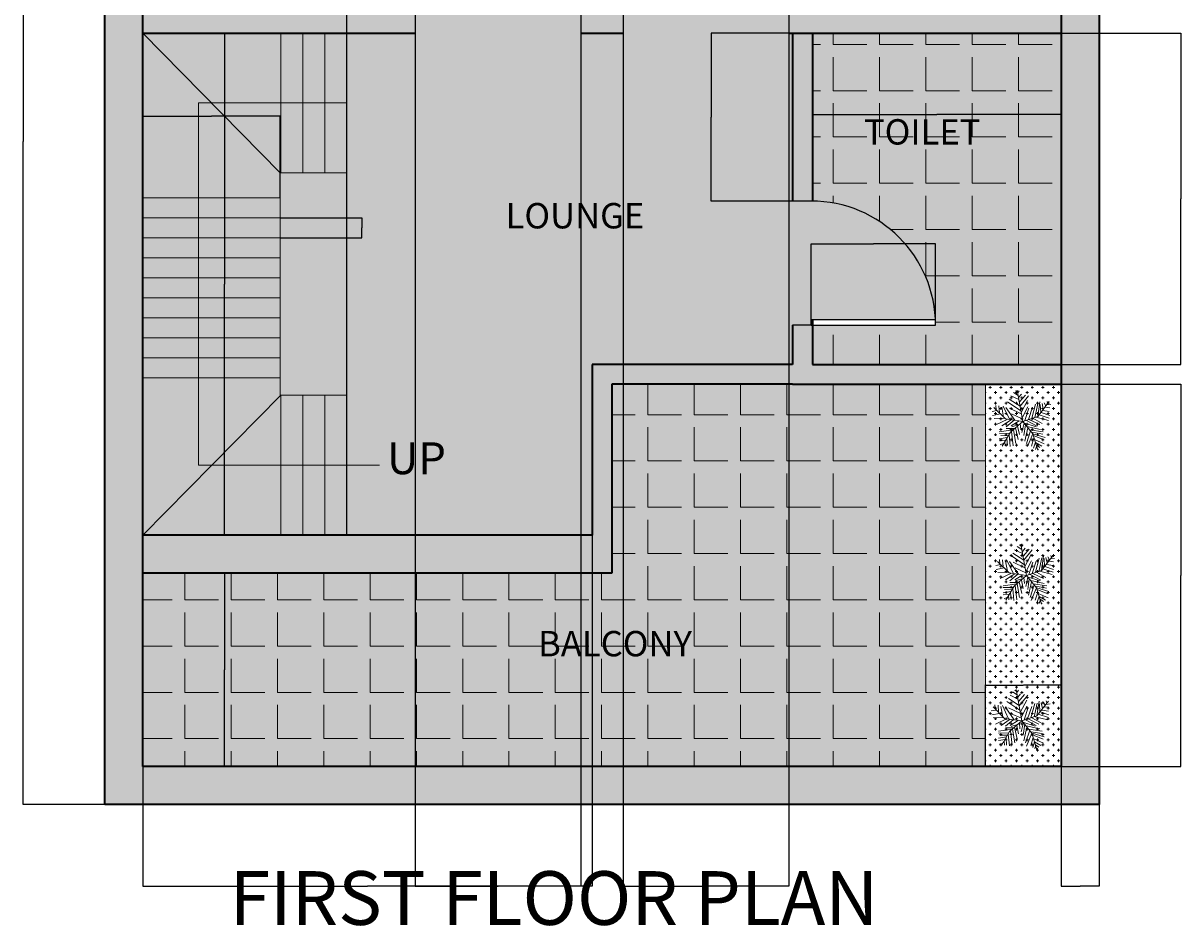
# Model space of a CAD drawing. Units: millimetres. Extents: x 1166 to 16630, y -7192 to 2820.
# Tile 7 of 8: x 9646 to 16630, y -6412 to -963. Entities that reach past the tile are written whole.
import ezdxf

# ---------------------------------------------------------------- set-up
doc = ezdxf.new("R2010")
doc.units = ezdxf.units.MM
for name, color, linetype, lineweight in [('A-ANNO-DIMS', 2, 'Continuous', 18), ('A-ANNO-SYMB', 7, 'Continuous', 18), ('A-ANNO-TEXT', 7, 'Continuous', 35), ('A-AREA-IDEN', 7, 'Continuous', 18), ('A-DOOR', 4, 'Continuous', 25), ('A-FLOR-PATT', 8, 'Continuous', 13), ('A-FLOR-STRS', 7, 'Continuous', 18), ('A-WALL', 7, 'Continuous', 35), ('L-PLNT', 70, 'Continuous', 18), ('L-PLNT-PATT', 3, 'Continuous', 13)]:
    doc.layers.add(name, color=color, linetype=linetype, lineweight=lineweight)
doc.layers.add('A-FLOR-FNSH-PATT', color=254, linetype='Continuous', lineweight=13, true_color=0xfeeab9)
doc.layers.add('A-WALL-PATT', color=254, linetype='Continuous', lineweight=13, true_color=0xcecce6)
doc.styles.get("Standard").update_dxf_attribs({"font": 'arial.ttf'})
doc.dimstyles.get("Standard").update_dxf_attribs({"dimtxt": 0.18, "dimasz": 0.18, "dimexe": 0.18, "dimexo": 0.0625, "dimgap": 0.09, "dimtad": 0, "dimtih": 1, "dimtoh": 1, "dimdec": 4, "dimzin": 0, "dimdsep": 46, "dimtxsty": 'Standard', "dimcen": 0.09, "dimadec": 0, "dimazin": 0, "dimtfac": 1, "dimtdec": 4, "dimtofl": 0, "dimtmove": 0, "dimatfit": 3, "dimfxl": 1, "dimtolj": 1, "dimtzin": 0, "dimarcsym": 0})
pattern_1 = [(0, (-8657.52, -11987.85), (0, 279.4), [203.2, -76.2]), (90, (-8657.52, -11987.85), (-279.4, 2e-14), [203.2, -76.2])]

# ---------------------------------------------------------------- blocks, each defined once
blk = doc.blocks.new('*U2')
for p, q in [((0, 0), (0, 6)), ((40, 0), (40, 6))]:
    blk.add_line(p, q)
blk.add_lwpolyline([(0, 0), (0, -40), (1.75, -40), (1.75, 0)], close=True)
blk.add_arc((0, 0), 40, 270, 0)
blk = doc.blocks.new('*U12')
for p, q in [((-7.288, 39.707), (-21.778, 46.673)), ((-8.737, 47.138), (-17.069, 52.711)), ((-10.186, 53.64), (-13.084, 55.962)), ((0, 0), (-10.5, 57)), ((-9.099, 51.782), (-6.563, 55.962)), ((-7.65, 43.423), (-2.578, 49.46)), ((-5.839, 35.992), (4.667, 48.067)), ((-5.114, 27.632), (10.463, 46.673)), ((-31.5, 4.5), (-52.5, 25.5)), ((-48.585, 21.131), (-49.309, 29.026)), ((-43.513, 28.561), (-42.427, 15.558)), ((-38.442, 26.239), (-34.819, 7.663)), ((-35.544, 28.097), (-24.314, 3.947)), ((-14.533, 2.09), (-30.834, 25.31)), ((-3.665, 19.273), (-27.574, 35.527)), ((-5.114, 28.097), (-24.676, 40.636)), ((-24.314, 23.917), (-2.941, 13.7)), ((-2.941, 16.486), (8.652, 37.85)), ((-1.129, 6.734), (9.014, 26.704)), ((3.942, 1.625), (11.187, 24.381)), ((10.101, 3.483), (17.708, 26.239)), ((16.259, 5.805), (23.142, 31.348)), ((22.055, 7.198), (27.489, 32.277)), ((27, 9), (48, 36)), ((27.127, 9.056), (31.112, 35.992)), ((31.836, 30.883), (32.561, 16.486)), ((35.096, 32.741), (37.27, 22.524)), ((38.719, 34.134), (41.979, 28.561)), ((40.53, 25.775), (48.862, 24.846)), ((43.791, 29.954), (51.036, 30.883)), ((44.153, 36.456), (45.239, 32.741)), ((-47.498, 19.737), (-55.83, 18.344)), ((-40.615, 13.7), (-55.105, 10.913)), ((-33.37, 6.269), (-52.207, 5.34)), ((-28.299, 3.483), (-47.86, -5.805)), ((-21.416, 3.018), (-38.079, -8.128)), ((0, 0), (-31.5, 4.5)), ((-15.982, 2.09), (-30.11, -9.521)), ((0, 0), (-22.5, -19.5)), ((-6.563, 1.161), (-21.416, -8.128)), ((-20.691, 13.7), (-1.129, 4.876)), ((0, 0), (27, 9)), ((0, 0), (18, -22.5)), ((6.478, 1.625), (26.04, -8.592)), ((11.187, 3.483), (30.749, -5.805)), ((18.07, 5.805), (35.096, -3.483)), ((24.229, 7.663), (46.688, 1.625)), ((29.662, 12.307), (48.137, 6.269)), ((33.285, 16.486), (48.862, 10.913)), ((36.183, 19.737), (48.137, 17.88)), ((-17.431, -15.094), (-42.789, -18.809)), ((-22.5, -19.5), (-37.5, -45)), ((-15.257, -12.772), (-30.11, -12.772)), ((-20.691, -18.345), (-17.793, -44.352)), ((-6.563, -5.805), (-19.967, -9.985)), ((-17.069, -15.094), (-12.721, -40.172)), ((-13.446, -11.378), (-8.737, -32.741)), ((-9.461, -8.592), (-6.201, -23.453)), ((-4.752, -3.483), (-3.665, -14.629)), ((2.493, -3.019), (-1.491, -20.202)), ((1.769, -2.555), (24.229, -9.521)), ((5.029, -6.27), (2.131, -25.775)), ((9.014, -11.378), (3.58, -35.992)), ((14.085, -16.951), (6.478, -40.172)), ((7.565, -9.056), (32.198, -14.629)), ((12.274, -15.094), (36.907, -18.809)), ((16.259, -19.738), (36.183, -22.989)), ((-28.299, -29.026), (-42.789, -31.348)), ((-24.314, -21.596), (-42.427, -22.06)), ((-30.834, -34.135), (-42.427, -35.528)), ((-34.457, -39.708), (-40.978, -42.494)), ((-26.849, -26.24), (-40.253, -25.775)), ((-32.646, -36.921), (-31.921, -44.352)), ((-29.023, -30.884), (-27.936, -43.887)), ((-25.038, -23.918), (-22.865, -45.281)), ((18.07, -22.524), (8.289, -45.745)), ((20.244, -30.419), (15.897, -44.816)), ((18, -22.5), (27, -52.5)), ((18.433, -22.524), (40.53, -29.026)), ((19.157, -25.311), (38.719, -33.206)), ((22.78, -37.85), (19.519, -48.532)), ((21.331, -32.741), (39.081, -40.636)), ((22.78, -38.314), (34.372, -44.816)), ((24.591, -45.745), (23.142, -50.854)), ((24.591, -43.423), (30.749, -47.603)), ((26.764, -49.925), (28.213, -50.854))]:
    blk.add_line(p, q)
blk = doc.blocks.new('*D49')
at = {"layer": 'A-ANNO-DIMS', "color": 0, "lineweight": -2, "transparency": 16777216}
for p, q in [((10138.1, 2327.5), (9646, 2327.5)), ((9646.2, 2327.3), (9646.2, -1676.3)), ((9646.2, -5680.2), (9646.2, -1676.6)), ((10138.1, -5680.3), (9646, -5680.3))]:
    blk.add_line(p, q, dxfattribs=at)
at = {"layer": 'A-ANNO-DIMS', "color": 0, "transparency": 16777216}
for points in [[(9646.2, 2327.3), (9646.2, 2327.3), (9646.2, 2327.5)], [(9646.2, -5680.2), (9646.2, -5680.2), (9646.2, -5680.3)]]:
    blk.add_solid(points, dxfattribs=at)
at = {"layer": 'Defpoints', "color": 0, "transparency": 16777216}
for p in [(10138.2, 2327.5), (9646.2, -5680.3), (10138.2, -5680.3)]:
    blk.add_point(p, dxfattribs=at)
at = {"layer": 'A-ANNO-DIMS', "color": 0, "transparency": 16777216, "insert": (9646.2, -1676.4), "char_height": 0.18, "attachment_point": 5}
blk.add_mtext('\\A1;8008', dxfattribs=at)
blk = doc.blocks.new('*D53')
at = {"layer": 'A-ANNO-DIMS', "color": 0, "lineweight": -2, "transparency": 16777216}
for p, q in [((10368.3, -1022.5), (10860.4, -1022.5)), ((10860.2, -1022.7), (10860.2, -2537.6)), ((10860.2, -4052.8), (10860.2, -2537.9)), ((10368.3, -4053), (10860.4, -4053))]:
    blk.add_line(p, q, dxfattribs=at)
at = {"layer": 'A-ANNO-DIMS', "color": 0, "transparency": 16777216}
for points in [[(10860.2, -1022.7), (10860.2, -1022.7), (10860.2, -1022.5)], [(10860.2, -4052.8), (10860.2, -4052.8), (10860.2, -4053)]]:
    blk.add_solid(points, dxfattribs=at)
at = {"layer": 'Defpoints', "color": 0, "transparency": 16777216}
for p in [(10368.2, -1022.5), (10368.2, -4053), (10860.2, -4053)]:
    blk.add_point(p, dxfattribs=at)
at = {"layer": 'A-ANNO-DIMS', "color": 0, "transparency": 16777216, "insert": (10860.2, -2537.8), "char_height": 0.18, "attachment_point": 5}
blk.add_mtext('\\A1;3030.4', dxfattribs=at)
blk = doc.blocks.new('*D54')
at = {"layer": 'A-ANNO-DIMS', "color": 0, "lineweight": -2, "transparency": 16777216}
for p, q in [((10368.206606, -4053.037033), (10368.206606, -6172.523929)), ((13078.206606, -4053.037033), (13078.206606, -6172.523929)), ((10368.386606, -6172.343929), (11722.846606, -6172.343929)), ((13078.026606, -6172.343929), (11723.566606, -6172.343929))]:
    blk.add_line(p, q, dxfattribs=at)
at = {"layer": 'A-ANNO-DIMS', "color": 0, "transparency": 16777216}
for points in [[(10368.386606, -6172.313929), (10368.386606, -6172.373929), (10368.206606, -6172.343929)], [(13078.026606, -6172.313929), (13078.026606, -6172.373929), (13078.206606, -6172.343929)]]:
    blk.add_solid(points, dxfattribs=at)
at = {"layer": 'Defpoints', "color": 0, "transparency": 16777216}
for p in [(10368.206606, -4052.974533), (13078.206606, -4052.974533), (13078.206606, -6172.343929)]:
    blk.add_point(p, dxfattribs=at)
at = {"layer": 'A-ANNO-DIMS', "color": 0, "transparency": 16777216, "insert": (11723.206606, -6172.343929), "char_height": 0.18, "attachment_point": 5}
blk.add_mtext('\\A1;2710', dxfattribs=at)
blk = doc.blocks.new('*D55')
at = {"layer": 'A-ANNO-DIMS', "color": 0, "lineweight": -2, "transparency": 16777216}
for p, q in [((14408.2, -1022.6), (14408.2, -1514.7)), ((15908.2, -1022.6), (15908.2, -1514.7)), ((14408.4, -1514.5), (15157.9, -1514.5)), ((15908, -1514.5), (15158.6, -1514.5))]:
    blk.add_line(p, q, dxfattribs=at)
at = {"layer": 'A-ANNO-DIMS', "color": 0, "transparency": 16777216}
for points in [[(14408.4, -1514.5), (14408.4, -1514.6), (14408.2, -1514.5)], [(15908, -1514.5), (15908, -1514.6), (15908.2, -1514.5)]]:
    blk.add_solid(points, dxfattribs=at)
at = {"layer": 'Defpoints', "color": 0, "transparency": 16777216}
for p in [(14408.2, -1022.5), (15908.2, -1022.5), (14408.2, -1514.5)]:
    blk.add_point(p, dxfattribs=at)
at = {"layer": 'A-ANNO-DIMS', "color": 0, "transparency": 16777216, "insert": (15158.2, -1514.5), "char_height": 0.18, "attachment_point": 5}
blk.add_mtext('\\A1;1500', dxfattribs=at)
blk = doc.blocks.new('*D56')
at = {"layer": 'A-ANNO-DIMS', "color": 0, "lineweight": -2, "transparency": 16777216}
for p, q in [((15908.3, -1022.5), (16630.4, -1022.5)), ((16630.2, -1022.7), (16630.2, -2022.4)), ((16630.2, -3022.4), (16630.2, -2022.7)), ((15908.3, -3022.5), (16630.4, -3022.5))]:
    blk.add_line(p, q, dxfattribs=at)
at = {"layer": 'A-ANNO-DIMS', "color": 0, "transparency": 16777216}
for points in [[(16630.2, -1022.7), (16630.2, -1022.7), (16630.2, -1022.5)], [(16630.2, -3022.4), (16630.2, -3022.4), (16630.2, -3022.5)]]:
    blk.add_solid(points, dxfattribs=at)
at = {"layer": 'Defpoints', "color": 0, "transparency": 16777216}
for p in [(15908.2, -1022.5), (15908.2, -3022.5), (16630.2, -3022.5)]:
    blk.add_point(p, dxfattribs=at)
at = {"layer": 'A-ANNO-DIMS', "color": 0, "transparency": 16777216, "insert": (16630.2, -2022.5), "char_height": 0.18, "attachment_point": 5}
blk.add_mtext('\\A1;2000', dxfattribs=at)
blk = doc.blocks.new('*D57')
at = {"layer": 'A-ANNO-DIMS', "color": 0, "lineweight": -2, "transparency": 16777216}
for p, q in [((15908.3, -3142.5), (16630.4, -3142.5)), ((16630.2, -3142.7), (16630.2, -4296.3)), ((16630.2, -5450.2), (16630.2, -4296.6)), ((15908.3, -5450.3), (16630.4, -5450.3))]:
    blk.add_line(p, q, dxfattribs=at)
at = {"layer": 'A-ANNO-DIMS', "color": 0, "transparency": 16777216}
for points in [[(16630.2, -3142.7), (16630.2, -3142.7), (16630.2, -3142.5)], [(16630.2, -5450.2), (16630.2, -5450.2), (16630.2, -5450.3)]]:
    blk.add_solid(points, dxfattribs=at)
at = {"layer": 'Defpoints', "color": 0, "transparency": 16777216}
for p in [(15908.2, -3142.5), (15908.2, -5450.3), (16630.2, -5450.3)]:
    blk.add_point(p, dxfattribs=at)
at = {"layer": 'A-ANNO-DIMS', "color": 0, "transparency": 16777216, "insert": (16630.2, -4296.4), "char_height": 0.18, "attachment_point": 5}
blk.add_mtext('\\A1;2308', dxfattribs=at)
blk = doc.blocks.new('*D58')
at = {"layer": 'A-ANNO-DIMS', "color": 0, "lineweight": -2, "transparency": 16777216}
for p, q in [((10368.3, -4283), (10860.4, -4283)), ((10860.2, -4283.2), (10860.2, -4866.5)), ((10860.2, -5450.2), (10860.2, -4866.8)), ((10368.3, -5450.3), (10860.4, -5450.3))]:
    blk.add_line(p, q, dxfattribs=at)
at = {"layer": 'A-ANNO-DIMS', "color": 0, "transparency": 16777216}
for points in [[(10860.2, -4283.2), (10860.2, -4283.2), (10860.2, -4283)], [(10860.2, -5450.2), (10860.2, -5450.2), (10860.2, -5450.3)]]:
    blk.add_solid(points, dxfattribs=at)
at = {"layer": 'Defpoints', "color": 0, "transparency": 16777216}
for p in [(10368.2, -4283), (10368.2, -5450.3), (10860.2, -5450.3)]:
    blk.add_point(p, dxfattribs=at)
at = {"layer": 'A-ANNO-DIMS', "color": 0, "transparency": 16777216, "insert": (10860.2, -4866.7), "char_height": 0.18, "attachment_point": 5}
blk.add_mtext('\\A1;1167.4', dxfattribs=at)
blk = doc.blocks.new('*D59')
at = {"layer": 'A-ANNO-DIMS', "color": 0, "lineweight": -2, "transparency": 16777216}
for p, q in [((12011.1, -902.6), (12011.1, -6172.5)), ((13011.1, -902.6), (13011.1, -6172.5)), ((12011.3, -6172.3), (12510.8, -6172.3)), ((13010.9, -6172.3), (12511.5, -6172.3))]:
    blk.add_line(p, q, dxfattribs=at)
at = {"layer": 'A-ANNO-DIMS', "color": 0, "transparency": 16777216}
for points in [[(12011.3, -6172.3), (12011.3, -6172.4), (12011.1, -6172.3)], [(13010.9, -6172.3), (13010.9, -6172.4), (13011.1, -6172.3)]]:
    blk.add_solid(points, dxfattribs=at)
at = {"layer": 'Defpoints', "color": 0, "transparency": 16777216}
for p in [(12011.1, -902.5), (13011.1, -902.5), (13011.1, -6172.3)]:
    blk.add_point(p, dxfattribs=at)
at = {"layer": 'A-ANNO-DIMS', "color": 0, "transparency": 16777216, "insert": (12511.1, -6172.3), "char_height": 0.18, "attachment_point": 5}
blk.add_mtext('\\A1;1000', dxfattribs=at)
blk = doc.blocks.new('*D60')
at = {"layer": 'A-ANNO-DIMS', "color": 0, "lineweight": -2, "transparency": 16777216}
for p, q in [((13265.3, -902.6), (13265.3, -6172.5)), ((14265.3, -902.6), (14265.3, -6172.5)), ((13265.5, -6172.3), (13765, -6172.3)), ((14265.1, -6172.3), (13765.7, -6172.3))]:
    blk.add_line(p, q, dxfattribs=at)
at = {"layer": 'A-ANNO-DIMS', "color": 0, "transparency": 16777216}
for points in [[(13265.5, -6172.3), (13265.5, -6172.4), (13265.3, -6172.3)], [(14265.1, -6172.3), (14265.1, -6172.4), (14265.3, -6172.3)]]:
    blk.add_solid(points, dxfattribs=at)
at = {"layer": 'Defpoints', "color": 0, "transparency": 16777216}
for p in [(13265.3, -902.5), (14265.3, -902.5), (14265.3, -6172.3)]:
    blk.add_point(p, dxfattribs=at)
at = {"layer": 'A-ANNO-DIMS', "color": 0, "transparency": 16777216, "insert": (13765.3, -6172.3), "char_height": 0.18, "attachment_point": 5}
blk.add_mtext('\\A1;1000', dxfattribs=at)
blk = doc.blocks.new('*D61')
at = {"layer": 'A-ANNO-DIMS', "color": 0, "lineweight": -2, "transparency": 16777216}
for p, q in [((14400.7, -2786.5), (14400.7, -2294.4)), ((14400.9, -2294.6), (14775.4, -2294.6)), ((15150.5, -2294.6), (14776, -2294.6)), ((15150.7, -2786.5), (15150.7, -2294.4))]:
    blk.add_line(p, q, dxfattribs=at)
at = {"layer": 'A-ANNO-DIMS', "color": 0, "transparency": 16777216}
for points in [[(14400.9, -2294.5), (14400.9, -2294.6), (14400.7, -2294.6)], [(15150.5, -2294.5), (15150.5, -2294.6), (15150.7, -2294.6)]]:
    blk.add_solid(points, dxfattribs=at)
at = {"layer": 'Defpoints', "color": 0, "transparency": 16777216}
for p in [(15150.7, -2294.6), (14400.7, -2786.6), (15150.7, -2786.6)]:
    blk.add_point(p, dxfattribs=at)
at = {"layer": 'A-ANNO-DIMS', "color": 0, "transparency": 16777216, "insert": (14775.7, -2294.6), "char_height": 0.18, "attachment_point": 5}
blk.add_mtext('\\A1;750', dxfattribs=at)
blk = doc.blocks.new('*D62')
at = {"layer": 'A-ANNO-DIMS', "color": 0, "lineweight": -2, "transparency": 16777216}
for p, q in [((10368.2, -4052.9), (10368.2, 2819.6)), ((10368.4, 2819.5), (10982.9, 2819.5)), ((11598.3, 2819.5), (10983.8, 2819.5)), ((11598.5, -4052.9), (11598.5, 2819.6))]:
    blk.add_line(p, q, dxfattribs=at)
at = {"layer": 'A-ANNO-DIMS', "color": 0, "transparency": 16777216}
for points in [[(10368.4, 2819.5), (10368.4, 2819.4), (10368.2, 2819.5)], [(11598.3, 2819.5), (11598.3, 2819.4), (11598.5, 2819.5)]]:
    blk.add_solid(points, dxfattribs=at)
at = {"layer": 'Defpoints', "color": 0, "transparency": 16777216}
for p in [(11598.5, 2819.5), (10368.2, -4053), (11598.5, -4053)]:
    blk.add_point(p, dxfattribs=at)
at = {"layer": 'A-ANNO-DIMS', "color": 0, "transparency": 16777216, "insert": (10983.4, 2819.5), "char_height": 0.18, "attachment_point": 5}
blk.add_mtext('\\A1;1230.3', dxfattribs=at)
blk = doc.blocks.new('*D63')
at = {"layer": 'A-ANNO-DIMS', "color": 0, "lineweight": -2, "transparency": 16777216}
for p, q in [((15908.2, -5450.4), (15908.2, -6172.5)), ((16138.2, -5680.4), (16138.2, -6172.5)), ((15908.4, -6172.3), (16022.9, -6172.3)), ((16138, -6172.3), (16023.5, -6172.3))]:
    blk.add_line(p, q, dxfattribs=at)
at = {"layer": 'A-ANNO-DIMS', "color": 0, "transparency": 16777216}
for points in [[(15908.4, -6172.3), (15908.4, -6172.4), (15908.2, -6172.3)], [(16138, -6172.3), (16138, -6172.4), (16138.2, -6172.3)]]:
    blk.add_solid(points, dxfattribs=at)
at = {"layer": 'Defpoints', "color": 0, "transparency": 16777216}
for p in [(15908.2, -5450.3), (16138.2, -5680.3), (15908.2, -6172.3)]:
    blk.add_point(p, dxfattribs=at)
at = {"layer": 'A-ANNO-DIMS', "color": 0, "transparency": 16777216, "insert": (16023.2, -6172.3), "char_height": 0.18, "attachment_point": 5}
blk.add_mtext('\\A1;230', dxfattribs=at)
blk = doc.blocks.new('*D64')
at = {"layer": 'A-ANNO-DIMS', "color": 0, "lineweight": -2, "transparency": 16777216}
for p, q in [((15452.3, -5450.3), (15452.3, -4958.2)), ((15452.5, -4958.3), (15679.9, -4958.3)), ((15908, -4958.3), (15680.7, -4958.3)), ((15908.2, -5450.3), (15908.2, -4958.2))]:
    blk.add_line(p, q, dxfattribs=at)
at = {"layer": 'A-ANNO-DIMS', "color": 0, "transparency": 16777216}
for points in [[(15452.5, -4958.3), (15452.5, -4958.4), (15452.3, -4958.3)], [(15908, -4958.3), (15908, -4958.4), (15908.2, -4958.3)]]:
    blk.add_solid(points, dxfattribs=at)
at = {"layer": 'Defpoints', "color": 0, "transparency": 16777216}
for p in [(15908.2, -4958.3), (15452.3, -5450.3), (15908.2, -5450.3)]:
    blk.add_point(p, dxfattribs=at)
at = {"layer": 'A-ANNO-DIMS', "color": 0, "transparency": 16777216, "insert": (15680.3, -4958.3), "char_height": 0.18, "attachment_point": 5}
blk.add_mtext('\\A1;455.9', dxfattribs=at)
blk = doc.blocks.new('*D66')
at = {"layer": 'A-ANNO-DIMS', "color": 0, "lineweight": -2, "transparency": 16777216}
for p, q in [((14288.1, -1022.5), (13796, -1022.5)), ((13796.2, -1022.7), (13796.2, -1529.4)), ((13796.2, -2036.4), (13796.2, -1529.7)), ((14288.1, -2036.6), (13796, -2036.6))]:
    blk.add_line(p, q, dxfattribs=at)
at = {"layer": 'A-ANNO-DIMS', "color": 0, "transparency": 16777216}
for points in [[(13796.2, -1022.7), (13796.2, -1022.7), (13796.2, -1022.5)], [(13796.2, -2036.4), (13796.2, -2036.4), (13796.2, -2036.6)]]:
    blk.add_solid(points, dxfattribs=at)
at = {"layer": 'Defpoints', "color": 0, "transparency": 16777216}
for p in [(13796.2, -1022.5), (14288.2, -1022.5), (14288.2, -2036.6)]:
    blk.add_point(p, dxfattribs=at)
at = {"layer": 'A-ANNO-DIMS', "color": 0, "transparency": 16777216, "insert": (13796.2, -1529.5), "char_height": 0.18, "attachment_point": 5}
blk.add_mtext('\\A1;1014', dxfattribs=at)
blk = doc.blocks.new('*D67')
at = {"layer": 'A-ANNO-DIMS', "color": 0, "lineweight": -2, "transparency": 16777216}
for p, q in [((10368.2, -2016.9), (10368.2, -1524.7)), ((10368.4, -1524.9), (10781.9, -1524.9)), ((11196.1, -1524.9), (10782.5, -1524.9)), ((11196.3, -2016.9), (11196.3, -1524.7))]:
    blk.add_line(p, q, dxfattribs=at)
at = {"layer": 'A-ANNO-DIMS', "color": 0, "transparency": 16777216}
for points in [[(10368.4, -1524.9), (10368.4, -1524.9), (10368.2, -1524.9)], [(11196.1, -1524.9), (11196.1, -1524.9), (11196.3, -1524.9)]]:
    blk.add_solid(points, dxfattribs=at)
at = {"layer": 'Defpoints', "color": 0, "transparency": 16777216}
for p in [(11196.3, -1524.9), (10368.2, -2016.9), (11196.3, -2016.9)]:
    blk.add_point(p, dxfattribs=at)
at = {"layer": 'A-ANNO-DIMS', "color": 0, "transparency": 16777216, "insert": (10782.2, -1524.9), "char_height": 0.18, "attachment_point": 5}
blk.add_mtext('\\A1;828', dxfattribs=at)
blk = doc.blocks.new('*D68')
at = {"layer": 'A-ANNO-DIMS', "color": 0, "lineweight": -2, "transparency": 16777216}
for p, q in [((11196.3, -2137.7), (11688.4, -2137.7)), ((11688.3, -2137.8), (11688.3, -2197.8)), ((11688.3, -2258.2), (11688.3, -2198.2)), ((11196.3, -2258.4), (11688.4, -2258.4))]:
    blk.add_line(p, q, dxfattribs=at)
at = {"layer": 'A-ANNO-DIMS', "color": 0, "transparency": 16777216}
for points in [[(11688.2, -2137.8), (11688.3, -2137.8), (11688.3, -2137.7)], [(11688.2, -2258.2), (11688.3, -2258.2), (11688.3, -2258.4)]]:
    blk.add_solid(points, dxfattribs=at)
at = {"layer": 'Defpoints', "color": 0, "transparency": 16777216}
for p in [(11196.3, -2137.7), (11196.3, -2258.4), (11688.3, -2258.4)]:
    blk.add_point(p, dxfattribs=at)
at = {"layer": 'A-ANNO-DIMS', "color": 0, "transparency": 16777216, "insert": (11688.3, -2198), "char_height": 0.18, "attachment_point": 5}
blk.add_mtext('\\A1;120.74', dxfattribs=at)

msp = doc.modelspace()

# ---------------------------------------------------------------- hatches: boundary and pattern name
at = {"layer": 'A-FLOR-FNSH-PATT', "transparency": 33554549}
h = msp.add_hatch(color=256, dxfattribs=at)
h.dxf.hatch_style = 1
h.paths.add_polyline_path([(14288.207, -1022.538), (14265.313, -1022.538), (14265.313, -872.538, 0.40145271), (13309.063, 126.505), (13309.063, -872.538), (13265.313, -872.538), (13265.313, -1022.538), (13011.1, -1022.538), (13011.1, -872.538), (12967.35, -872.538), (12967.35, 126.505, 0.40145271), (12011.1, -872.538), (12011.1, -1022.538), (11598.503, -1022.538), (11598.503, -1865.538), (11598.503, -3209.099), (11598.503, -4052.975), (13078.207, -4052.975), (13078.207, -3022.538), (14288.207, -3022.538), (14288.207, -2786.562), (14400.707, -2786.562), (14400.707, -2753.749), (15149.988, -2753.749, 0.40145271), (14400.707, -2036.562), (14288.207, -2036.562)])
h.paths.add_polyline_path([(11598.503, -1865.538), (11196.269, -1865.538), (11196.269, -3209.099), (11598.503, -3209.099)])
h.paths.add_polyline_path([(13078.207, 2097.462), (10368.207, 2097.462), (10368.207, -902.538), (12011.1, -902.538), (12011.1, -872.538, -0.40145271), (12967.35, 126.505), (12967.35, 127.462), (13011.1, 127.462), (13011.1, -872.538), (13011.1, -902.538), (13078.207, -902.538)])
h.paths.add_polyline_path([(11836.742, 538.355), (10431.54, 538.355), (10431.54, 1592.256), (11836.742, 1592.256)], flags=16)
h.paths.add_polyline_path([(10951.465, 538.355), (10719.606, 770.213), (10719.606, 678.875), (10452.618, 678.875), (10452.618, 1044.228), (10684.476, 1044.228), (10684.476, 1086.384), (10452.618, 1086.384), (10452.618, 1451.736), (10684.476, 1451.736), (10684.476, 805.343), (10951.465, 805.343)], flags=16)
h.paths.add_polyline_path([(15908.207, 2097.462), (13198.207, 2097.462), (13198.207, 847.342), (13214.293, 863.428), (13214.293, 1474.722), (13503.853, 1474.722), (13503.853, 1426.462), (13519.94, 1426.462), (13519.94, 1233.422), (13503.853, 1233.422), (13503.853, 1217.335), (13519.94, 1217.335), (13519.94, 1024.295), (13503.853, 1024.295), (13503.853, 976.035), (13519.94, 976.035), (13519.94, 959.948, -0.09090909), (13519.94, 606.042), (13519.94, 589.955), (13503.853, 589.955), (13503.853, 509.522), (13214.293, 509.522), (13214.293, 702.562), (13198.207, 718.648), (13198.207, -902.538), (13265.313, -902.538), (13265.313, -872.538), (13265.313, 127.462), (13309.063, 127.462), (13309.063, 126.505, -0.40145271), (14265.313, -872.538), (14265.313, -902.538), (15908.207, -902.538)])
h.paths.add_polyline_path([(14427.327, 538.355), (14427.327, 1592.256), (15832.53, 1592.256), (15832.53, 538.355)], flags=16)
h.paths.add_polyline_path([(15312.605, 538.355), (15312.605, 805.343), (15579.593, 805.343), (15579.593, 1451.736), (15811.452, 1451.736), (15811.452, 1086.384), (15579.593, 1086.384), (15579.593, 1044.228), (15811.452, 1044.228), (15811.452, 678.875), (15544.463, 678.875), (15544.463, 770.213)], flags=16)
h.paths.add_polyline_path([(12516.729, -2244.054), (13499.854, -2244.054), (13499.854, -2006.254), (12516.729, -2006.254)], flags=24)
h.paths.add_polyline_path([(11791.983, -3737.781), (12263.574, -3737.781), (12263.574, -3444.03), (11791.983, -3444.03)], flags=24)
h.paths.add_polyline_path([(10753.982, -293.014), (11939.114, -293.014), (11939.114, -55.214), (10753.982, -55.214)], flags=24)
h.paths.add_polyline_path([(14420.893, -296.216), (15606.026, -296.216), (15606.026, -58.416), (14420.893, -58.416)], flags=24)
h = msp.add_hatch(color=256, dxfattribs=at)
h.dxf.hatch_style = 1
h.paths.add_polyline_path([(11199.893, -1022.538), (10368.207, -1022.538), (10782.238, -1444.038), (11199.893, -1444.038)])
h.paths.add_polyline_path([(11332.763, -1022.538), (11199.893, -1022.538), (11199.893, -1444.038), (11332.763, -1444.038)])
h.paths.add_polyline_path([(11465.633, -1022.538), (11332.763, -1022.538), (11332.763, -1444.038), (11465.633, -1444.038)])
h.paths.add_polyline_path([(11598.503, -1022.538), (11465.633, -1022.538), (11465.633, -1444.038), (11598.503, -1444.038)])
h.paths.add_polyline_path([(11598.503, -1444.038), (11465.633, -1444.038), (11465.633, -1865.538), (11598.503, -1865.538)])
h.paths.add_polyline_path([(11465.633, -1444.038), (11332.763, -1444.038), (11332.763, -1865.538), (11465.633, -1865.538)])
h.paths.add_polyline_path([(11332.763, -1444.038), (11199.893, -1444.038), (11199.893, -1865.538), (11332.763, -1865.538)])
h.paths.add_polyline_path([(11199.893, -1444.038), (10782.238, -1444.038), (11196.269, -1865.538), (11199.893, -1865.538)])
h.paths.add_polyline_path([(10704.756, -1444.038), (10782.238, -1444.038), (10368.207, -1022.538), (10368.207, -2016.918), (10704.756, -2016.918)])
h.paths.add_polyline_path([(10782.238, -1444.038), (10704.756, -1444.038), (10704.756, -2016.918), (11196.269, -2016.918), (11196.269, -1865.538)])
h.paths.add_polyline_path([(11196.269, -2016.918), (10704.756, -2016.918), (10704.756, -2137.658), (11196.269, -2137.658)])
h.paths.add_polyline_path([(11196.269, -2137.658), (10704.756, -2137.658), (10704.756, -2258.398), (11196.269, -2258.398)])
h.paths.add_polyline_path([(11196.269, -2258.398), (10704.756, -2258.398), (10704.756, -2379.138), (11196.269, -2379.138)])
h.paths.add_polyline_path([(11196.269, -2379.138), (10704.756, -2379.138), (10704.756, -2499.878), (11196.269, -2499.878)])
h.paths.add_polyline_path([(11196.269, -2499.878), (10704.756, -2499.878), (10704.756, -2620.619), (11196.269, -2620.619)])
h.paths.add_polyline_path([(11196.269, -2620.619), (10704.756, -2620.619), (10704.756, -2741.359), (11196.269, -2741.359)])
h.paths.add_polyline_path([(11196.269, -2741.359), (10704.756, -2741.359), (10704.756, -2862.099), (11196.269, -2862.099)])
h.paths.add_polyline_path([(11196.269, -2862.099), (10704.756, -2862.099), (10704.756, -2982.839), (11196.269, -2982.839)])
h.paths.add_polyline_path([(11196.269, -2982.839), (10704.756, -2982.839), (10704.756, -3103.579), (11196.269, -3103.579)])
h.paths.add_polyline_path([(10704.756, -2982.839), (10368.207, -2982.839), (10368.207, -3103.579), (10704.756, -3103.579)])
h.paths.add_polyline_path([(10704.756, -2862.099), (10368.207, -2862.099), (10368.207, -2982.839), (10704.756, -2982.839)])
h.paths.add_polyline_path([(10704.756, -2741.359), (10368.207, -2741.359), (10368.207, -2862.099), (10704.756, -2862.099)])
h.paths.add_polyline_path([(10704.756, -2620.619), (10368.207, -2620.619), (10368.207, -2741.359), (10704.756, -2741.359)])
h.paths.add_polyline_path([(10704.756, -2499.878), (10368.207, -2499.878), (10368.207, -2620.619), (10704.756, -2620.619)])
h.paths.add_polyline_path([(10704.756, -2379.138), (10368.207, -2379.138), (10368.207, -2499.878), (10704.756, -2499.878)])
h.paths.add_polyline_path([(10704.756, -2258.398), (10368.207, -2258.398), (10368.207, -2379.138), (10704.756, -2379.138)])
h.paths.add_polyline_path([(10704.756, -2016.918), (10368.207, -2016.918), (10368.207, -2137.658), (10704.756, -2137.658)])
h.paths.add_polyline_path([(10704.756, -2137.658), (10368.207, -2137.658), (10368.207, -2258.398), (10704.756, -2258.398)])
h.paths.add_polyline_path([(11199.893, -3209.099), (11196.269, -3209.099), (11196.269, -3103.579), (10704.756, -3103.579), (10704.756, -3631.037), (10784.05, -3631.037)])
h.paths.add_polyline_path([(10704.756, -3103.579), (10368.207, -3103.579), (10368.207, -4052.975), (10784.05, -3631.037), (10704.756, -3631.037)])
h.paths.add_polyline_path([(11199.893, -3209.099), (10784.05, -3631.037), (11199.893, -3631.037)], flags=17)
h.paths.add_polyline_path([(11199.893, -3631.037), (10784.05, -3631.037), (10368.207, -4052.975), (11199.893, -4052.975)])
h.paths.add_polyline_path([(11332.763, -3209.099), (11199.893, -3209.099), (11199.893, -3631.037), (11332.763, -3631.037)])
h.paths.add_polyline_path([(11465.633, -3209.099), (11332.763, -3209.099), (11332.763, -3631.037), (11465.633, -3631.037)])
h.paths.add_polyline_path([(11598.503, -3209.099), (11465.633, -3209.099), (11465.633, -3631.037), (11598.503, -3631.037)])
h.paths.add_polyline_path([(11598.503, -3631.037), (11465.633, -3631.037), (11465.633, -4052.975), (11598.503, -4052.975)])
h.paths.add_polyline_path([(11465.633, -3631.037), (11332.763, -3631.037), (11332.763, -4052.975), (11465.633, -4052.975)])
h.paths.add_polyline_path([(11332.763, -3631.037), (11199.893, -3631.037), (11199.893, -4052.975), (11332.763, -4052.975)])
at = {"layer": 'A-FLOR-FNSH-PATT', "transparency": 33554574}
h = msp.add_hatch(color=256, dxfattribs=at)
h.dxf.hatch_style = 1
h.paths.add_polyline_path([(15908.207, -1022.538), (14408.207, -1022.538), (14408.207, -2036.599, -0.39855266), (15149.988, -2753.749), (15150.707, -2753.749), (15150.707, -2786.562), (14408.207, -2786.562), (14408.207, -3022.538), (15908.207, -3022.538)])
h.paths.add_polyline_path([(14678.782, -1737.829), (15507.241, -1737.829), (15507.241, -1500.03), (14678.782, -1500.03)], flags=24)
at = {"layer": 'A-FLOR-FNSH-PATT', "transparency": 33554549}
h = msp.add_hatch(color=256, dxfattribs=at)
h.dxf.hatch_style = 1
h.paths.add_polyline_path([(15452.336, -3142.538), (14288.207, -3142.538), (13198.207, -3142.538), (13198.207, -4282.975), (10368.207, -4282.975), (10368.207, -5450.344), (15452.336, -5450.344)])
h.paths.add_polyline_path([(12712.811, -4827.516), (13814.967, -4827.516), (13814.967, -4589.717), (12712.811, -4589.717)], flags=24)
at = {"layer": 'A-FLOR-PATT', "transparency": 33554546}
h = msp.add_hatch(dxfattribs=at)
h.set_pattern_fill('ANGLE', color=256, scale=40)
h.set_pattern_definition(pattern_1)
h.paths.add_polyline_path([(15908.207, -1022.538), (14408.207, -1022.538), (14408.207, -2036.599, -0.39855266), (15149.988, -2753.749), (15150.707, -2753.749), (15150.707, -2786.562), (14408.207, -2786.562), (14408.207, -3022.538), (15908.207, -3022.538)])
h.paths.add_polyline_path([(14678.782, -1737.829), (15507.241, -1737.829), (15507.241, -1500.03), (14678.782, -1500.03)], flags=24)
h = msp.add_hatch(dxfattribs=at)
h.set_pattern_fill('ANGLE', color=256, scale=40)
h.set_pattern_definition(pattern_1)
h.paths.add_polyline_path([(15452.336, -3142.538), (14288.207, -3142.538), (13198.207, -3142.538), (13198.207, -4282.975), (10368.207, -4282.975), (10368.207, -5450.344), (15452.336, -5450.344)])
h.paths.add_polyline_path([(12712.811, -4827.516), (13814.967, -4827.516), (13814.967, -4589.717), (12712.811, -4589.717)], flags=24)
at = {"layer": 'A-WALL-PATT'}
h = msp.add_hatch(color=256, dxfattribs=at)
h.dxf.hatch_style = 1
h.paths.add_polyline_path([(10138.207, 2327.462), (10138.207, -5680.344), (16138.207, -5680.344), (16138.207, 2327.462)])
h.paths.add_polyline_path([(15908.207, 2097.462), (15908.207, -5450.344), (10368.207, -5450.344), (10368.207, 2097.462)], flags=16)
h.paths.add_polyline_path([(14427.327, 1592.256), (15832.53, 1592.256), (15832.53, 538.355), (14427.327, 538.355)], flags=0)
h.paths.add_polyline_path([(15579.593, 805.343), (15579.593, 1451.736), (15811.452, 1451.736), (15811.452, 1086.384), (15579.593, 1086.384), (15579.593, 1044.228), (15811.452, 1044.228), (15811.452, 678.875), (15544.463, 678.875), (15544.463, 770.213), (15312.605, 538.355), (15312.605, 805.343)], flags=0)
h.paths.add_polyline_path([(11598.503, -1022.538), (11598.503, -1865.538), (11598.503, -3209.099), (11598.503, -4052.099), (11598.503, -4052.975), (10368.207, -4052.975), (10784.05, -3631.037), (10704.756, -3631.037), (10704.756, -1444.038), (10782.238, -1444.038), (10368.207, -1022.538)], flags=0)
h.paths.add_polyline_path([(12967.35, 127.462), (13011.1, 127.462), (13011.1, -872.538), (12967.35, -872.538)], flags=0)
h.paths.add_polyline_path([(12712.811, -4827.516), (13814.967, -4827.516), (13814.967, -4589.717), (12712.811, -4589.717)], flags=8)
h.paths.add_polyline_path([(12516.729, -2244.054), (13499.854, -2244.054), (13499.854, -2006.254), (12516.729, -2006.254)], flags=8)
h.paths.add_polyline_path([(14678.782, -1737.829), (15507.241, -1737.829), (15507.241, -1500.03), (14678.782, -1500.03)], flags=8)
h.paths.add_polyline_path([(14420.893, -296.216), (15606.026, -296.216), (15606.026, -58.416), (14420.893, -58.416)], flags=8)
h.paths.add_polyline_path([(10753.982, -293.014), (11939.114, -293.014), (11939.114, -55.214), (10753.982, -55.214)], flags=8)
h.paths.add_polyline_path([(11791.983, -3737.781), (12263.574, -3737.781), (12263.574, -3444.03), (11791.983, -3444.03)], flags=8)
h = msp.add_hatch(color=256, dxfattribs=at)
h.dxf.hatch_style = 1
h.paths.add_polyline_path([(13198.207, -3142.538), (14288.207, -3142.538), (15908.207, -3142.538), (15908.207, -3022.538), (14408.207, -3022.538), (14408.207, -2786.562), (14400.707, -2786.562), (14288.207, -2786.562), (14288.207, -3022.538), (13078.207, -3022.538), (13078.207, -4052.975), (10368.207, -4052.975), (10368.207, -4282.975), (13198.207, -4282.975)])
h.paths.add_polyline_path([(12011.1, -902.538), (10368.207, -902.538), (10368.207, -1022.538), (12011.1, -1022.538)])
h.paths.add_polyline_path([(13198.207, 2097.462), (13078.207, 2097.462), (13078.207, -902.538), (13198.207, -902.538)])
h.paths.add_polyline_path([(15908.207, -902.538), (14265.313, -902.538), (14265.313, -1022.538), (15908.207, -1022.538)])
h.paths.add_polyline_path([(14408.207, -1022.538), (14288.207, -1022.538), (14288.207, -2036.562), (14408.207, -2036.562)])
h.paths.add_polyline_path([(13265.313, -902.538), (13011.1, -902.538), (13011.1, -1022.538), (13265.313, -1022.538)])
at = {"layer": 'L-PLNT-PATT'}
h = msp.add_hatch(dxfattribs=at)
h.set_pattern_fill('CROSS', color=256, scale=5)
h.set_pattern_definition([(0, (-8657.52, -11987.852), (31.75, 31.75), [15.875, -47.625]), (90, (-8649.582, -11995.79), (-31.75, 31.75), [15.875, -47.625])])
h.paths.add_polyline_path([(15908.207, -3142.538), (15452.336, -3142.538), (15452.336, -5450.344), (15908.207, -5450.344)])

# ---------------------------------------------------------------- linework, layer by layer
at = {"layer": 'A-ANNO-SYMB'}
for p, q in [((11598.503, -1444.038), (10704.756, -1444.038)), ((10704.756, -1444.038), (10704.756, -3631.037)), ((10704.756, -3631.037), (11794.835, -3631.037))]:
    msp.add_line(p, q, dxfattribs=at)
at = {"layer": 'A-FLOR-STRS', "transparency": 33554554}
for p, q in [((11196.269, -1865.538), (10368.207, -1022.538)), ((11199.893, -1865.538), (11199.893, -1022.538)), ((11332.763, -1865.538), (11332.763, -1022.538)), ((11465.633, -1865.538), (11465.633, -1022.538)), ((11598.503, -1865.538), (11598.503, -1022.538)), ((11598.503, -1865.538), (11598.503, -3209.099)), ((11196.269, -2016.918), (10368.207, -2016.918)), ((11196.269, -2137.658), (10368.207, -2137.658)), ((11196.269, -2258.398), (10368.207, -2258.398)), ((11196.269, -2379.138), (10368.207, -2379.138)), ((11196.269, -2499.878), (10368.207, -2499.878)), ((11196.269, -2620.619), (10368.207, -2620.619)), ((11196.269, -2741.359), (10368.207, -2741.359)), ((11196.269, -2862.099), (10368.207, -2862.099)), ((11196.269, -2982.839), (10368.207, -2982.839)), ((11196.269, -3103.579), (10368.207, -3103.579)), ((11199.893, -3209.099), (10368.207, -4052.975)), ((11199.893, -3209.099), (11199.893, -4052.099)), ((11332.763, -3209.099), (11332.763, -4052.099)), ((11465.633, -3209.099), (11465.633, -4052.099)), ((11598.503, -3209.099), (11598.503, -4052.975)), ((11598.503, -3209.099), (11598.503, -4052.099))]:
    msp.add_line(p, q, dxfattribs=at)
msp.add_lwpolyline([(11598.503, -3209.099), (11196.269, -3209.099), (11196.269, -1865.538), (11598.503, -1865.538)], dxfattribs=at)
at = {"layer": 'A-WALL'}
for p, q in [((10138.207, -5680.344), (10138.207, 2327.462)), ((16138.207, 2327.462), (16138.207, -5680.344)), ((10368.207, -5450.344), (10368.207, 2097.462)), ((15908.207, 2097.462), (15908.207, -5450.344)), ((10368.207, -1022.538), (12011.1, -1022.538)), ((13011.1, -1022.538), (13265.313, -1022.538)), ((14265.313, -1022.538), (15908.207, -1022.538)), ((14288.207, -1022.538), (14288.207, -2036.562)), ((14408.207, -1022.538), (14408.207, -2036.599)), ((14288.207, -2786.562), (14288.207, -3022.538)), ((14408.207, -2753.749), (14408.207, -3022.538)), ((14288.207, -3022.538), (13078.207, -3022.538)), ((13078.207, -3022.538), (13078.207, -4052.975)), ((14408.207, -3022.538), (15908.207, -3022.538)), ((14288.207, -3142.538), (13198.207, -3142.538)), ((13198.207, -3142.538), (13198.207, -4282.975)), ((14288.207, -3142.538), (15908.207, -3142.538)), ((13078.207, -4052.975), (10368.207, -4052.975)), ((13198.207, -4282.975), (10368.207, -4282.975)), ((15908.207, -5450.344), (10368.207, -5450.344)), ((16138.207, -5680.344), (10138.207, -5680.344))]:
    msp.add_line(p, q, dxfattribs=at)
at = {"layer": 'L-PLNT'}
msp.add_line((15452.336, -3142.538), (15452.336, -5450.344), dxfattribs=at)

# ---------------------------------------------------------------- block references
at = {"layer": 'A-DOOR'}
for p, xscale, yscale, zscale, rotation in [((13011.1, -872.538), 25, 25, 25, 180), ((13265.313, -872.538), -25, 25, 25, 180), ((14400.707, -2786.562), 18.75, 18.75, 18.75, 90)]:
    msp.add_blockref('*U2', p, dxfattribs=dict(at, xscale=xscale, yscale=yscale, zscale=zscale, rotation=rotation))
at = {"layer": 'L-PLNT', "xscale": 3.318952487250034, "yscale": 3.318952487250034, "zscale": 3.318952487250034}
for p in [(15677.08, -3367.223), (15699.562, -4296.959), (15672.105, -5174.874)]:
    msp.add_blockref('*U12', p, dxfattribs=at)

# ---------------------------------------------------------------- texts
at = {"layer": 'A-ANNO-SYMB'}
msp.add_text('UP', height=192.5506, dxfattribs=at).set_placement((11840.941, -3685.539))
at = {"layer": 'A-ANNO-TEXT'}
msp.add_text('FIRST FLOOR PLAN', height=324.44434, dxfattribs=at).set_placement((10890.926, -6406.604))
at = {"layer": 'A-AREA-IDEN'}
for s, p in [('TOILET', (14718.416, -1695.583)), ('LOUNGE', (12556.362, -2201.808)), ('BALCONY', (12752.444, -4785.27))]:
    msp.add_text(s, height=153.2035, dxfattribs=at).set_placement(p)

# ---------------------------------------------------------------- dimensions: what is measured, and where the dimension line sits
at = {"layer": 'A-ANNO-DIMS'}
for base, p1, p2, override, picture, middle in [((11598.503, 2819.462), (10368.207, -4052.975), (11598.503, -4052.975), {"dimdec": 1, "dimlfac": 1, "dimrnd": 0, "dimzin": 0, "dimdsep": 46, "dimlunit": 2}, '*D62', (10983.355, 2819.462)), ((13011.1, -6172.344), (12011.1, -902.538), (13011.1, -902.538), {"dimdec": 0, "dimlfac": 1, "dimrnd": 0, "dimzin": 0, "dimdsep": 46, "dimlunit": 2}, '*D59', (12511.1, -6172.344)), ((14265.313, -6172.344), (13265.313, -902.538), (14265.313, -902.538), {"dimdec": 0, "dimlfac": 1, "dimrnd": 0, "dimzin": 0, "dimdsep": 46, "dimlunit": 2}, '*D60', (13765.313, -6172.344)), ((11196.269, -1524.918), (10368.207, -2016.918), (11196.269, -2016.918), {"dimdec": 0, "dimlfac": 1, "dimrnd": 0, "dimzin": 0, "dimdsep": 46, "dimlunit": 2}, '*D67', (10782.238, -1524.918)), ((15150.707, -2294.562), (14400.707, -2786.562), (15150.707, -2786.562), {"dimdec": 0, "dimlfac": 1, "dimrnd": 0, "dimzin": 0, "dimdsep": 46, "dimlunit": 2}, '*D61', (14775.707, -2294.562)), ((13078.207, -6172.344), (10368.207, -4052.975), (13078.207, -4052.975), {"dimdec": 0, "dimlfac": 1, "dimrnd": 0, "dimzin": 0, "dimdsep": 46, "dimlunit": 2}, '*D54', (11723.207, -6172.344)), ((15908.207, -4958.344), (15452.336, -5450.344), (15908.207, -5450.344), {"dimdec": 1, "dimlfac": 1, "dimrnd": 0, "dimzin": 0, "dimdsep": 46, "dimlunit": 2}, '*D64', (15680.272, -4958.344)), ((15908.207, -6172.344), (16138.207, -5680.344), (15908.207, -5450.344), {"dimdec": 0, "dimlfac": 1, "dimrnd": 0, "dimzin": 0, "dimdsep": 46, "dimlunit": 2}, '*D63', (16023.207, -6172.344))]:
    dim = msp.add_linear_dim(base=base, p1=p1, p2=p2, dimstyle='Standard', override=override, dxfattribs=at)
    dim.commit()
    dim.dimension.update_dxf_attribs({"geometry": picture, "text_midpoint": middle})
for base, p1, p2, angle, override, picture, middle in [((9646.207, -5680.344), (10138.207, 2327.462), (10138.207, -5680.344), 90, {"dimdec": 0, "dimlfac": 1, "dimrnd": 0, "dimzin": 0, "dimdsep": 46, "dimlunit": 2}, '*D49', (9646.207, -1676.441)), ((10860.207, -4052.975), (10368.207, -1022.538), (10368.207, -4052.975), 270, {"dimdec": 1, "dimlfac": 1, "dimrnd": 0, "dimzin": 0, "dimdsep": 46, "dimlunit": 2}, '*D53', (10860.207, -2537.756)), ((13796.207, -1022.538), (14288.207, -2036.562), (14288.207, -1022.538), 90, {"dimdec": 0, "dimlfac": 1, "dimrnd": 0, "dimzin": 0, "dimdsep": 46, "dimlunit": 2}, '*D66', (13796.207, -1529.55)), ((14408.207, -1514.538), (15908.207, -1022.538), (14408.207, -1022.538), 180, {"dimdec": 0, "dimlfac": 1, "dimrnd": 0, "dimzin": 0, "dimdsep": 46, "dimlunit": 2}, '*D55', (15158.207, -1514.538)), ((16630.207, -3022.538), (15908.207, -1022.538), (15908.207, -3022.538), 90, {"dimdec": 0, "dimlfac": 1, "dimrnd": 0, "dimzin": 0, "dimdsep": 46, "dimlunit": 2}, '*D56', (16630.207, -2022.538)), ((11688.269, -2258.398), (11196.269, -2137.658), (11196.269, -2258.398), 270, {"dimdec": 2, "dimlfac": 1, "dimrnd": 0, "dimzin": 0, "dimdsep": 46, "dimlunit": 2}, '*D68', (11688.269, -2198.028)), ((16630.207, -5450.344), (15908.207, -3142.538), (15908.207, -5450.344), 90, {"dimdec": 0, "dimlfac": 1, "dimrnd": 0, "dimzin": 0, "dimdsep": 46, "dimlunit": 2}, '*D57', (16630.207, -4296.441)), ((10860.207, -5450.344), (10368.207, -4282.975), (10368.207, -5450.344), 270, {"dimdec": 1, "dimlfac": 1, "dimrnd": 0, "dimzin": 0, "dimdsep": 46, "dimlunit": 2}, '*D58', (10860.207, -4866.659))]:
    dim = msp.add_linear_dim(base=base, p1=p1, p2=p2, angle=angle, dimstyle='Standard', override=override, dxfattribs=at)
    dim.commit()
    dim.dimension.update_dxf_attribs({"geometry": picture, "text_midpoint": middle})

doc.saveas('drawing.dxf')
